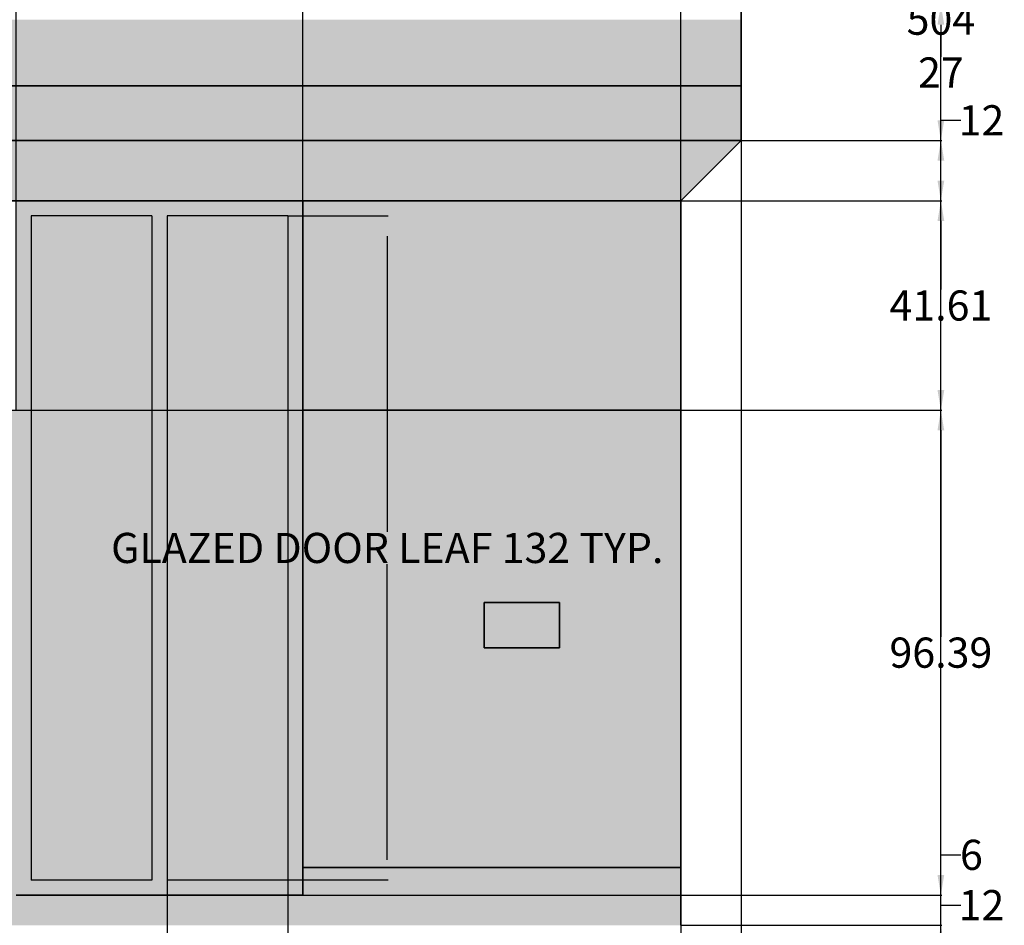
# Model space of a CAD drawing. Units: inches. Extents: x 221 to 874, y 171 to 738.
# Tile 10 of 11: x 650 to 845, y 275 to 455. Entities that reach past the tile are written whole.
import ezdxf

# ---------------------------------------------------------------- set-up
doc = ezdxf.new("R2010")
doc.units = ezdxf.units.IN
doc.header["$MEASUREMENT"] = 0
for name, color, linetype, lineweight in [('A-ANNO-DIMS', 2, 'Continuous', 18), ('A-DOOR', 4, 'Continuous', 25), ('A-ELEV', 7, 'Continuous', 35), ('A-ELEV-PATT', 8, 'Continuous', 13)]:
    doc.layers.add(name, color=color, linetype=linetype, lineweight=lineweight)
doc.styles.get("Standard").update_dxf_attribs({"font": 'arial.ttf'})
doc.dimstyles.get("Standard").update_dxf_attribs({"dimtxt": 6, "dimasz": 4, "dimexe": 0.18, "dimexo": 0.0625, "dimgap": 0.09, "dimtad": 0, "dimtih": 1, "dimtoh": 1, "dimdec": 0, "dimzin": 0, "dimdsep": 46, "dimlunit": 3, "dimtxsty": 'Standard', "dimcen": 0.09, "dimadec": 0, "dimazin": 0, "dimtfac": 1, "dimtdec": 0, "dimtofl": 0, "dimtmove": 0, "dimatfit": 3, "dimfxl": 1, "dimtolj": 1, "dimtzin": 0, "dimarcsym": 0})

# ---------------------------------------------------------------- blocks, each defined once
blk = doc.blocks.new('DOOR-LEAF-GLAZED')
for p, q in [((0, 132), (0, 0)), ((24, 132), (0, 132)), ((24, 132), (24, 0)), ((24, 0), (0, 0))]:
    blk.add_line(p, q)
blk = doc.blocks.new('*D12')
at = {"layer": 'A-ANNO-DIMS', "color": 0, "lineweight": -2, "transparency": 16777216}
for p, q in [((702.97, 415.72), (722.89, 415.72)), ((722.71, 411.72), (722.71, 352.91)), ((722.71, 287.72), (722.71, 346.52)), ((702.97, 283.72), (722.89, 283.72))]:
    blk.add_line(p, q, dxfattribs=at)
at = {"layer": 'A-ANNO-DIMS', "color": 0, "transparency": 16777216}
for points in [[(722.04, 411.72), (723.38, 411.72), (722.71, 415.72)], [(722.04, 287.72), (723.38, 287.72), (722.71, 283.72)]]:
    blk.add_solid(points, dxfattribs=at)
at = {"layer": 'Defpoints', "color": 0, "transparency": 16777216}
for p in [(702.91, 415.72), (722.71, 415.72), (702.91, 283.72)]:
    blk.add_point(p, dxfattribs=at)
at = {"layer": 'A-ANNO-DIMS', "color": 0, "transparency": 16777216, "insert": (722.71, 349.72), "char_height": 6, "attachment_point": 5}
blk.add_mtext('\\A1;GLAZED DOOR LEAF 132 TYP.', dxfattribs=at)
blk = doc.blocks.new('*D13')
at = {"layer": 'A-ANNO-DIMS', "color": 0, "lineweight": -2, "transparency": 16777216}
for p, q in [((678.91, 283.65), (678.91, 263.74)), ((702.91, 283.65), (702.91, 263.74)), ((682.91, 263.92), (698.91, 263.92)), ((702.91, 263.92), (706.91, 263.92))]:
    blk.add_line(p, q, dxfattribs=at)
at = {"layer": 'A-ANNO-DIMS', "color": 0, "transparency": 16777216}
for points in [[(682.91, 264.58), (682.91, 263.25), (678.91, 263.92)], [(698.91, 264.58), (698.91, 263.25), (702.91, 263.92)]]:
    blk.add_solid(points, dxfattribs=at)
at = {"layer": 'Defpoints', "color": 0, "transparency": 16777216}
for p in [(678.91, 283.72), (702.91, 283.72), (702.91, 263.92)]:
    blk.add_point(p, dxfattribs=at)
at = {"layer": 'A-ANNO-DIMS', "color": 0, "transparency": 16777216, "insert": (721.65, 263.92), "char_height": 6, "attachment_point": 5}
blk.add_mtext('\\A1;24 TYP.', dxfattribs=at)
blk = doc.blocks.new('*D21')
at = {"layer": 'A-ANNO-DIMS', "color": 0, "lineweight": -2, "transparency": 16777216}
for p, q in [((541.14, 706.72), (833.01, 706.72)), ((832.83, 702.72), (832.83, 457.87)), ((832.83, 206.72), (832.83, 451.56)), ((805.14, 202.72), (833.01, 202.72))]:
    blk.add_line(p, q, dxfattribs=at)
at = {"layer": 'A-ANNO-DIMS', "color": 0, "transparency": 16777216}
for points in [[(832.16, 702.72), (833.5, 702.72), (832.83, 706.72)], [(832.16, 206.72), (833.5, 206.72), (832.83, 202.72)]]:
    blk.add_solid(points, dxfattribs=at)
at = {"layer": 'Defpoints', "color": 0, "transparency": 16777216}
for p in [(541.08, 706.72), (832.83, 706.72), (805.08, 202.72)]:
    blk.add_point(p, dxfattribs=at)
at = {"layer": 'A-ANNO-DIMS', "color": 0, "transparency": 16777216, "insert": (832.83, 454.72), "char_height": 6, "attachment_point": 5}
blk.add_mtext('\\A1;504', dxfattribs=at)
blk = doc.blocks.new('*D46')
at = {"layer": 'A-ANNO-DIMS', "color": 0, "lineweight": -2, "transparency": 16777216}
for p, q in [((793.08, 430.65), (793.08, 174.79)), ((781.08, 418.65), (781.08, 174.79)), ((785.08, 174.97), (789.08, 174.97)), ((793.08, 174.97), (797.08, 174.97))]:
    blk.add_line(p, q, dxfattribs=at)
at = {"layer": 'A-ANNO-DIMS', "color": 0, "transparency": 16777216}
for points in [[(785.08, 175.63), (785.08, 174.3), (781.08, 174.97)], [(789.08, 175.63), (789.08, 174.3), (793.08, 174.97)]]:
    blk.add_solid(points, dxfattribs=at)
at = {"layer": 'Defpoints', "color": 0, "transparency": 16777216}
for p in [(793.08, 430.72), (781.08, 418.72), (793.08, 174.97)]:
    blk.add_point(p, dxfattribs=at)
at = {"layer": 'A-ANNO-DIMS', "color": 0, "transparency": 16777216, "insert": (801.15, 174.97), "char_height": 6, "attachment_point": 5}
blk.add_mtext('\\A1;12', dxfattribs=at)
blk = doc.blocks.new('*D47')
at = {"layer": 'A-ANNO-DIMS', "color": 0, "lineweight": -2, "transparency": 16777216}
for p, q in [((832.83, 430.72), (832.83, 434.72)), ((832.83, 434.72), (836.83, 434.72)), ((793.14, 430.72), (833.01, 430.72)), ((832.83, 422.72), (832.83, 426.72)), ((781.14, 418.72), (833.01, 418.72))]:
    blk.add_line(p, q, dxfattribs=at)
at = {"layer": 'A-ANNO-DIMS', "color": 0, "transparency": 16777216}
for points in [[(832.16, 426.72), (833.5, 426.72), (832.83, 430.72)], [(832.16, 422.72), (833.5, 422.72), (832.83, 418.72)]]:
    blk.add_solid(points, dxfattribs=at)
at = {"layer": 'Defpoints', "color": 0, "transparency": 16777216}
for p in [(793.08, 430.72), (832.83, 430.72), (781.08, 418.72)]:
    blk.add_point(p, dxfattribs=at)
at = {"layer": 'A-ANNO-DIMS', "color": 0, "transparency": 16777216, "insert": (840.9, 434.72), "char_height": 6, "attachment_point": 5}
blk.add_mtext('\\A1;12', dxfattribs=at)
blk = doc.blocks.new('*D48')
at = {"layer": 'A-ANNO-DIMS', "color": 0, "lineweight": -2, "transparency": 16777216}
for p, q in [((793.14, 457.72), (833.01, 457.72)), ((832.83, 453.72), (832.83, 447.32)), ((832.83, 434.72), (832.83, 441.11)), ((793.14, 430.72), (833.01, 430.72))]:
    blk.add_line(p, q, dxfattribs=at)
at = {"layer": 'A-ANNO-DIMS', "color": 0, "transparency": 16777216}
for points in [[(832.16, 453.72), (833.5, 453.72), (832.83, 457.72)], [(832.16, 434.72), (833.5, 434.72), (832.83, 430.72)]]:
    blk.add_solid(points, dxfattribs=at)
at = {"layer": 'Defpoints', "color": 0, "transparency": 16777216}
for p in [(793.08, 457.72), (832.83, 457.72), (793.08, 430.72)]:
    blk.add_point(p, dxfattribs=at)
at = {"layer": 'A-ANNO-DIMS', "color": 0, "transparency": 16777216, "insert": (832.83, 444.22), "char_height": 6, "attachment_point": 5}
blk.add_mtext('\\A1;27', dxfattribs=at)
blk = doc.blocks.new('*D60')
at = {"layer": 'A-ANNO-DIMS', "color": 0, "lineweight": -2, "transparency": 16777216}
for p, q in [((648.91, 377.16), (648.91, 734.65)), ((652.91, 734.47), (673.02, 734.47)), ((701.91, 734.47), (681.8, 734.47)), ((705.91, 377.16), (705.91, 734.65))]:
    blk.add_line(p, q, dxfattribs=at)
at = {"layer": 'A-ANNO-DIMS', "color": 0, "transparency": 16777216}
for points in [[(652.91, 735.13), (652.91, 733.8), (648.91, 734.47)], [(701.91, 735.13), (701.91, 733.8), (705.91, 734.47)]]:
    blk.add_solid(points, dxfattribs=at)
at = {"layer": 'Defpoints', "color": 0, "transparency": 16777216}
for p in [(705.91, 734.47), (648.91, 377.1), (705.91, 377.1)]:
    blk.add_point(p, dxfattribs=at)
at = {"layer": 'A-ANNO-DIMS', "color": 0, "transparency": 16777216, "insert": (677.41, 734.47), "char_height": 6, "attachment_point": 5}
blk.add_mtext('\\A1;57', dxfattribs=at)
blk = doc.blocks.new('*D61')
at = {"layer": 'A-ANNO-DIMS', "color": 0, "lineweight": -2, "transparency": 16777216}
for p, q in [((705.91, 377.16), (705.91, 734.65)), ((709.91, 734.47), (733.31, 734.47)), ((777.08, 734.47), (753.68, 734.47)), ((781.08, 377.16), (781.08, 734.65))]:
    blk.add_line(p, q, dxfattribs=at)
at = {"layer": 'A-ANNO-DIMS', "color": 0, "transparency": 16777216}
for points in [[(709.91, 735.13), (709.91, 733.8), (705.91, 734.47)], [(777.08, 735.13), (777.08, 733.8), (781.08, 734.47)]]:
    blk.add_solid(points, dxfattribs=at)
at = {"layer": 'Defpoints', "color": 0, "transparency": 16777216}
for p in [(781.08, 734.47), (705.91, 377.1), (781.08, 377.1)]:
    blk.add_point(p, dxfattribs=at)
at = {"layer": 'A-ANNO-DIMS', "color": 0, "transparency": 16777216, "insert": (743.49, 734.47), "char_height": 6, "attachment_point": 5}
blk.add_mtext('\\A1;75.17', dxfattribs=at)
blk = doc.blocks.new('*D63')
at = {"layer": 'A-ANNO-DIMS', "color": 0, "lineweight": -2, "transparency": 16777216}
for p, q in [((832.83, 274.72), (832.83, 278.72)), ((832.83, 278.72), (836.83, 278.72)), ((781.14, 274.72), (833.01, 274.72)), ((832.83, 266.72), (832.83, 270.72)), ((805.14, 262.72), (833.01, 262.72))]:
    blk.add_line(p, q, dxfattribs=at)
at = {"layer": 'A-ANNO-DIMS', "color": 0, "transparency": 16777216}
for points in [[(832.16, 270.72), (833.5, 270.72), (832.83, 274.72)], [(832.16, 266.72), (833.5, 266.72), (832.83, 262.72)]]:
    blk.add_solid(points, dxfattribs=at)
at = {"layer": 'Defpoints', "color": 0, "transparency": 16777216}
for p in [(781.08, 274.72), (832.83, 274.72), (805.08, 262.72)]:
    blk.add_point(p, dxfattribs=at)
at = {"layer": 'A-ANNO-DIMS', "color": 0, "transparency": 16777216, "insert": (840.9, 278.72), "char_height": 6, "attachment_point": 5}
blk.add_mtext('\\A1;12', dxfattribs=at)
blk = doc.blocks.new('*D64')
at = {"layer": 'A-ANNO-DIMS', "color": 0, "lineweight": -2, "transparency": 16777216}
for p, q in [((832.83, 284.72), (832.83, 288.72)), ((832.83, 288.72), (836.83, 288.72)), ((705.97, 280.72), (833.01, 280.72)), ((781.14, 274.72), (833.01, 274.72)), ((832.83, 270.72), (832.83, 266.72))]:
    blk.add_line(p, q, dxfattribs=at)
at = {"layer": 'A-ANNO-DIMS', "color": 0, "transparency": 16777216}
for points in [[(832.16, 284.72), (833.5, 284.72), (832.83, 280.72)], [(832.16, 270.72), (833.5, 270.72), (832.83, 274.72)]]:
    blk.add_solid(points, dxfattribs=at)
at = {"layer": 'Defpoints', "color": 0, "transparency": 16777216}
for p in [(705.91, 280.72), (832.83, 280.72), (781.08, 274.72)]:
    blk.add_point(p, dxfattribs=at)
at = {"layer": 'A-ANNO-DIMS', "color": 0, "transparency": 16777216, "insert": (838.9, 288.72), "char_height": 6, "attachment_point": 5}
blk.add_mtext('\\A1;6', dxfattribs=at)
blk = doc.blocks.new('*D65')
at = {"layer": 'A-ANNO-DIMS', "color": 0, "lineweight": -2, "transparency": 16777216}
for p, q in [((598.14, 377.1), (833.01, 377.1)), ((832.83, 373.1), (832.83, 332.06)), ((832.83, 284.72), (832.83, 325.75)), ((705.97, 280.72), (833.01, 280.72))]:
    blk.add_line(p, q, dxfattribs=at)
at = {"layer": 'A-ANNO-DIMS', "color": 0, "transparency": 16777216}
for points in [[(832.16, 373.1), (833.5, 373.1), (832.83, 377.1)], [(832.16, 284.72), (833.5, 284.72), (832.83, 280.72)]]:
    blk.add_solid(points, dxfattribs=at)
at = {"layer": 'Defpoints', "color": 0, "transparency": 16777216}
for p in [(598.08, 377.1), (832.83, 377.1), (705.91, 280.72)]:
    blk.add_point(p, dxfattribs=at)
at = {"layer": 'A-ANNO-DIMS', "color": 0, "transparency": 16777216, "insert": (832.83, 328.91), "char_height": 6, "attachment_point": 5}
blk.add_mtext('\\A1;96.39', dxfattribs=at)
blk = doc.blocks.new('*D66')
at = {"layer": 'A-ANNO-DIMS', "color": 0, "lineweight": -2, "transparency": 16777216}
for p, q in [((781.14, 418.72), (833.01, 418.72)), ((832.83, 414.72), (832.83, 401.06)), ((832.83, 381.1), (832.83, 394.76)), ((598.14, 377.1), (833.01, 377.1))]:
    blk.add_line(p, q, dxfattribs=at)
at = {"layer": 'A-ANNO-DIMS', "color": 0, "transparency": 16777216}
for points in [[(832.16, 414.72), (833.5, 414.72), (832.83, 418.72)], [(832.16, 381.1), (833.5, 381.1), (832.83, 377.1)]]:
    blk.add_solid(points, dxfattribs=at)
at = {"layer": 'Defpoints', "color": 0, "transparency": 16777216}
for p in [(781.08, 418.72), (832.83, 418.72), (598.08, 377.1)]:
    blk.add_point(p, dxfattribs=at)
at = {"layer": 'A-ANNO-DIMS', "color": 0, "transparency": 16777216, "insert": (832.83, 397.91), "char_height": 6, "attachment_point": 5}
blk.add_mtext('\\A1;41.61', dxfattribs=at)

msp = doc.modelspace()

# ---------------------------------------------------------------- hatches: boundary and pattern name
at = {"layer": 'A-ELEV-PATT'}
h = msp.add_hatch(color=256, dxfattribs=at)
h.dxf.hatch_style = 1
h.paths.add_polyline_path([(349.0786, 286.1996), (313.0786, 286.1996), (313.0786, 232.7164), (349.0786, 232.7164)])
h.paths.add_polyline_path([(464.0786, 286.1996), (406.0786, 286.1996), (406.0786, 232.7164), (464.0786, 232.7164)])
h.paths.add_polyline_path([(541.0786, 286.1996), (493.0786, 286.1996), (493.0786, 232.7164), (541.0786, 232.7164)])
h.paths.add_polyline_path([(541.0786, 370.7164), (493.0786, 370.7164), (493.0786, 286.1996), (541.0786, 286.1996)])
h.paths.add_polyline_path([(464.0786, 370.7164), (406.0786, 370.7164), (406.0786, 286.1996), (464.0786, 286.1996)])
h.paths.add_polyline_path([(349.0786, 370.7164), (313.0786, 370.7164), (313.0786, 286.1996), (349.0786, 286.1996)])
h.paths.add_polyline_path([(349.0786, 454.7164), (313.0786, 454.7164), (313.0786, 370.7164), (349.0786, 370.7164)])
h.paths.add_polyline_path([(464.0786, 454.7164), (406.0786, 454.7164), (406.0786, 370.7164), (464.0786, 370.7164)])
h.paths.add_polyline_path([(541.0786, 418.7164), (541.0786, 454.7164), (493.0786, 454.7164), (493.0786, 370.7164), (541.0786, 370.7164)])
h.paths.add_polyline_path([(541.0786, 550.7164), (493.0786, 550.7164), (493.0786, 454.7164), (541.0786, 454.7164)])
h.paths.add_polyline_path([(464.0786, 550.7164), (406.0786, 550.7164), (406.0786, 454.7164), (464.0786, 454.7164)])
h.paths.add_polyline_path([(349.0786, 550.7164), (313.0786, 550.7164), (313.0786, 454.7164), (349.0786, 454.7164)])
h.paths.add_polyline_path([(349.0786, 586.7164), (313.0786, 586.7164), (313.0786, 550.7164), (349.0786, 550.7164)])
h.paths.add_polyline_path([(464.0786, 586.7164), (406.0786, 586.7164), (406.0786, 550.7164), (464.0786, 550.7164)])
h.paths.add_polyline_path([(541.0786, 574.7164), (541.0786, 586.7164), (493.0786, 586.7164), (493.0786, 550.7164), (541.0786, 550.7164)])
h.paths.add_polyline_path([(541.0786, 670.7164), (493.0786, 670.7164), (493.0786, 586.7164), (541.0786, 586.7164)])
h.paths.add_polyline_path([(464.0786, 670.7164), (406.0786, 670.7164), (406.0786, 586.7164), (464.0786, 586.7164)])
h.paths.add_polyline_path([(349.0786, 670.7164), (313.0786, 670.7164), (313.0786, 586.7164), (349.0786, 586.7164)])
h.paths.add_polyline_path([(406.0786, 706.7164), (313.0786, 706.7164), (313.0786, 670.7164), (349.0786, 670.7164), (406.0786, 670.7164)])
h.paths.add_polyline_path([(464.0786, 706.7164), (406.0786, 706.7164), (406.0786, 670.7164), (464.0786, 670.7164)])
h.paths.add_polyline_path([(541.0786, 706.7164), (493.0786, 706.7164), (493.0786, 688.7164), (493.0786, 670.7164), (541.0786, 670.7164)])
h.paths.add_polyline_path([(660.0786, 610.7164), (541.0786, 610.7164), (541.0786, 586.7164), (541.0786, 574.7164), (660.0786, 574.7164)])
h.paths.add_polyline_path([(781.0786, 610.7164), (660.0786, 610.7164), (660.0786, 574.7164), (769.0786, 574.7164), (781.0786, 574.7164)])
h.paths.add_polyline_path([(781.0786, 574.7164), (769.0786, 574.7164), (769.0786, 476.1199), (781.0786, 476.1199)])
h.paths.add_polyline_path([(781.0786, 476.1199), (769.0786, 476.1199), (769.0786, 457.7164), (781.0786, 457.7164)])
h.paths.add_polyline_path([(781.0786, 377.1023), (705.9097, 377.1023), (705.9097, 286.1996), (781.0786, 286.1996)])
h.paths.add_polyline_path([(741.9618, 338.8486), (756.9618, 338.8486), (756.9618, 329.8486), (741.9618, 329.8486)], flags=16)
h.paths.add_polyline_path([(648.9097, 377.1023), (598.0786, 377.1023), (598.0786, 286.1996), (648.9097, 286.1996)])
h.paths.add_polyline_path([(781.0786, 286.1996), (705.9097, 286.1996), (705.9097, 280.7164), (648.9097, 280.7164), (648.9097, 286.1996), (598.0786, 286.1996), (598.0786, 280.7164), (550.0786, 280.7164), (550.0786, 286.1996), (541.0786, 286.1996), (541.0786, 274.7164), (781.0786, 274.7164)])
h.paths.add_polyline_path([(660.0786, 562.7164), (546.3477, 562.7164), (546.3477, 457.7164), (660.0786, 457.7164)])
h = msp.add_hatch(color=256, dxfattribs=at)
h.dxf.hatch_style = 1
h.paths.add_polyline_path([(793.0786, 441.595), (793.0786, 454.7164), (541.0786, 454.7164), (541.0786, 441.595)])
h = msp.add_hatch(color=256, dxfattribs=at)
h.dxf.hatch_style = 1
h.paths.add_polyline_path([(793.0786, 430.7164), (793.0786, 441.595), (541.0786, 441.595), (541.0786, 430.7164)])
h = msp.add_hatch(color=256, dxfattribs=at)
h.set_gradient(color1=(209, 204, 163), color2=(147, 149, 152), rotation=90, name='INVCYLINDER')
h.paths.add_polyline_path([(781.0786, 418.7164), (793.0786, 430.7164), (541.0786, 430.7164), (541.0786, 418.7164)])
h.paths.add_polyline_path([(587.5133, 425.0196, -1), (591.5133, 425.0196, -1)], flags=16)
h.paths.add_polyline_path([(557.7898, 425.0196, -1), (561.7898, 425.0196, -1)], flags=16)
h = msp.add_hatch(color=256, dxfattribs=at)
h.paths.add_polyline_path([(705.9097, 418.7164), (648.9097, 418.7164), (648.9097, 280.7164), (705.9097, 280.7164)])
h.paths.add_polyline_path([(675.9097, 415.7164), (675.9097, 283.7164), (651.9097, 283.7164), (651.9097, 415.7164)], flags=16)
h.paths.add_polyline_path([(678.9097, 415.7164), (702.9097, 415.7164), (702.9097, 283.7164), (678.9097, 283.7164)], flags=16)
h = msp.add_hatch(color=256, dxfattribs=at)
h.set_gradient(color1=(209, 204, 163), color2=(80, 81, 83), rotation=90)
h.paths.add_polyline_path([(781.0786, 377.1023), (781.0786, 418.7164), (705.9097, 418.7164), (705.9097, 377.1023)])
h = msp.add_hatch(color=256, dxfattribs=at)
h.set_gradient(color1=(254, 234, 185), color2=(237, 203, 135), name='INVSPHERICAL')
h.paths.add_polyline_path([(651.9097, 283.7164), (675.9097, 283.7164), (675.9097, 415.7164), (651.9097, 415.7164)])
h = msp.add_hatch(color=256, dxfattribs=at)
h.set_gradient(color1=(254, 234, 185), color2=(237, 203, 135), name='INVSPHERICAL')
h.paths.add_polyline_path([(702.9097, 415.7164), (678.9097, 415.7164), (678.9097, 283.7164), (702.9097, 283.7164)])
msp.add_hatch(color=256, dxfattribs=at).paths.add_polyline_path([(756.9618, 338.8486), (741.9618, 338.8486), (741.9618, 329.8486), (756.9618, 329.8486)])

# ---------------------------------------------------------------- linework, layer by layer
at = {"layer": 'A-ELEV'}
for p, q in [((793.0786, 457.7164), (793.0786, 430.7164)), ((541.0786, 441.595), (793.0786, 441.595)), ((793.0786, 430.7164), (541.0786, 430.7164)), ((781.0786, 418.7164), (793.0786, 430.7164)), ((781.0786, 418.7164), (541.0786, 418.7164)), ((705.9097, 418.7164), (705.9097, 280.7164)), ((781.0786, 418.7164), (781.0786, 274.7164)), ((705.9097, 377.1023), (781.0786, 377.1023)), ((741.9618, 338.8486), (756.9618, 338.8486)), ((741.9618, 329.8486), (741.9618, 338.8486)), ((756.9618, 338.8486), (756.9618, 329.8486)), ((756.9618, 329.8486), (741.9618, 329.8486)), ((705.9097, 286.1996), (781.0786, 286.1996)), ((705.9097, 280.7164), (648.9097, 280.7164))]:
    msp.add_line(p, q, dxfattribs=at)

# ---------------------------------------------------------------- block references
at = {"layer": 'A-DOOR'}
for p in [(651.91, 283.716), (678.91, 283.716)]:
    msp.add_blockref('DOOR-LEAF-GLAZED', p, dxfattribs=at)

# ---------------------------------------------------------------- dimensions: what is measured, and where the dimension line sits
at = {"layer": 'A-ANNO-DIMS'}
for base, p1, p2, override, picture, middle in [((705.9097, 734.4664), (648.9097, 377.1023), (705.9097, 377.1023), {"dimdec": 0, "dimlfac": 1, "dimrnd": 0, "dimzin": 0, "dimdsep": 46, "dimlunit": 2}, '*D60', (677.4097, 734.4664)), ((781.0786, 734.4664), (705.9097, 377.1023), (781.0786, 377.1023), {"dimdec": 2, "dimlfac": 1, "dimrnd": 0, "dimzin": 0, "dimdsep": 46, "dimlunit": 2}, '*D61', (743.4941, 734.4664)), ((793.0786, 174.9664), (781.0786, 418.7164), (793.0786, 430.7164), {"dimdec": 0, "dimlfac": 1, "dimrnd": 0, "dimzin": 0, "dimdsep": 46, "dimlunit": 2}, '*D46', (801.1529, 174.9664))]:
    dim = msp.add_linear_dim(base=base, p1=p1, p2=p2, dimstyle='Standard', override=override, dxfattribs=at)
    dim.commit()
    dim.dimension.update_dxf_attribs({"geometry": picture, "text_midpoint": middle})
for base, p1, p2, override, picture, middle in [((832.8286, 706.7164), (805.0786, 202.7164), (541.0786, 706.7164), {"dimdec": 0, "dimlfac": 1, "dimrnd": 0, "dimzin": 0, "dimdsep": 46, "dimlunit": 2}, '*D21', (832.8286, 454.7164)), ((832.8286, 457.7164), (793.0786, 430.7164), (793.0786, 457.7164), {"dimdec": 0, "dimlfac": 1, "dimrnd": 0, "dimzin": 0, "dimdsep": 46, "dimlunit": 2}, '*D48', (832.8286, 444.2164)), ((832.8286, 430.7164), (781.0786, 418.7164), (793.0786, 430.7164), {"dimdec": 0, "dimlfac": 1, "dimrnd": 0, "dimzin": 0, "dimdsep": 46, "dimlunit": 2}, '*D47', (840.9029, 434.7164)), ((832.8286, 418.7164), (598.0786, 377.1023), (781.0786, 418.7164), {"dimdec": 2, "dimlfac": 1, "dimrnd": 0, "dimzin": 0, "dimdsep": 46, "dimlunit": 2}, '*D66', (832.8286, 397.9093)), ((832.8286, 377.1023), (705.9097, 280.7164), (598.0786, 377.1023), {"dimdec": 2, "dimlfac": 1, "dimrnd": 0, "dimzin": 0, "dimdsep": 46, "dimlunit": 2}, '*D65', (832.8286, 328.9093)), ((832.8286, 280.7164), (781.0786, 274.7164), (705.9097, 280.7164), {"dimdec": 0, "dimlfac": 1, "dimrnd": 0, "dimzin": 0, "dimdsep": 46, "dimlunit": 2}, '*D64', (838.8995, 288.7164)), ((832.8286, 274.7164), (805.0786, 262.7164), (781.0786, 274.7164), {"dimdec": 0, "dimlfac": 1, "dimrnd": 0, "dimzin": 0, "dimdsep": 46, "dimlunit": 2}, '*D63', (840.9029, 278.7164))]:
    dim = msp.add_linear_dim(base=base, p1=p1, p2=p2, angle=90, dimstyle='Standard', override=override, dxfattribs=at)
    dim.commit()
    dim.dimension.update_dxf_attribs({"geometry": picture, "text_midpoint": middle})
dim = msp.add_linear_dim(base=(722.7097, 415.7164), p1=(702.9097, 283.7164), p2=(702.9097, 415.7164), angle=90, text='GLAZED DOOR LEAF <> TYP.', dimstyle='Standard', override={"dimdec": 0, "dimrnd": 0, "dimzin": 0, "dimlunit": 2}, dxfattribs=at)
dim.commit()
dim.dimension.update_dxf_attribs({"geometry": '*D12', "text_midpoint": (722.7097, 349.7164)})
dim = msp.add_linear_dim(base=(702.9097, 263.9164), p1=(678.9097, 283.7164), p2=(702.9097, 283.7164), text='<> TYP.', dimstyle='Standard', override={"dimdec": 0, "dimrnd": 0, "dimzin": 0, "dimlunit": 2}, dxfattribs=at)
dim.commit()
dim.dimension.update_dxf_attribs({"geometry": '*D13', "text_midpoint": (721.6538, 263.9164)})

doc.saveas('drawing.dxf')
